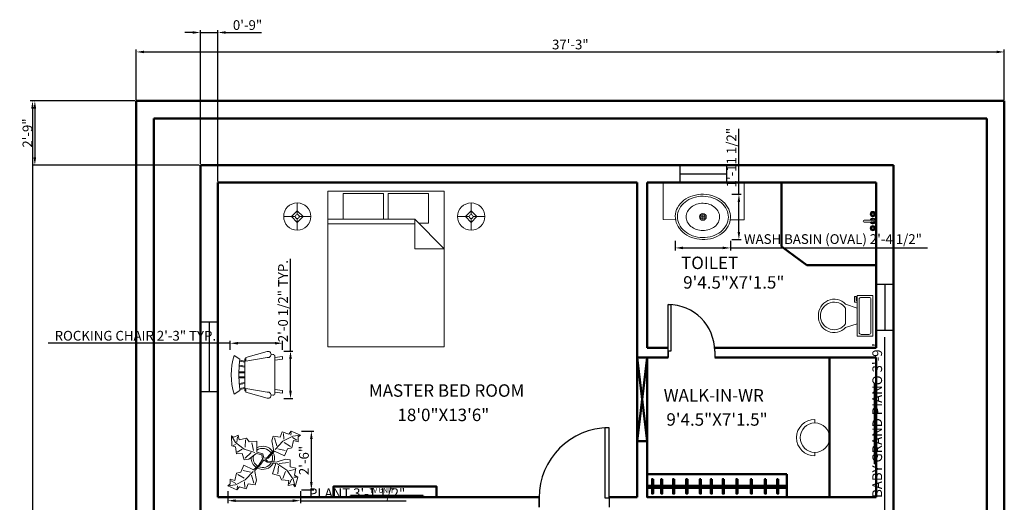
# Model space of a CAD drawing. Units: inches. Extents: x 116541 to 117938, y 135634 to 136328.
# Tile 9 of 9: x 117394 to 117902, y 136080 to 136328. Entities that reach past the tile are written whole.
import ezdxf

# ---------------------------------------------------------------- set-up
doc = ezdxf.new("R2010")
doc.units = ezdxf.units.IN
for name, color, linetype, lineweight in [('A-ANNO-DIMS', 2, 'Continuous', 18), ('A-ANNO-TEXT', 7, 'Continuous', 25), ('A-AREA-IDEN', 3, 'Continuous', 25), ('A-DOOR', 4, 'Continuous', 25), ('A-FLOR-FIXT', 9, 'Continuous', 18), ('A-FURN', 8, 'Continuous', 18), ('A-GLAZ', 1, 'Continuous', 25), ('A-WALL', 7, 'Continuous', 50)]:
    doc.layers.add(name, color=color, linetype=linetype, lineweight=lineweight)
doc.styles.get("Standard").update_dxf_attribs({"font": 'arial.ttf'})
doc.dimstyles.new('ISO-25', dxfattribs={"dimtxt": 5, "dimasz": 4, "dimexe": 1.25, "dimexo": 0.625, "dimtad": 1, "dimdec": 3, "dimlunit": 3, "dimtxsty": 'Standard', "dimcen": 2.5, "dimadec": 0, "dimazin": 0, "dimtfac": 1, "dimtdec": 3, "dimtmove": 0, "dimatfit": 3, "dimfxl": 1, "dimarcsym": 0})

# ---------------------------------------------------------------- blocks, each defined once
blk = doc.blocks.new('Plant - Rubber or Philodendron')
for p, q in [((-16.2005, 11.4774), (-13.9899, 8.1064)), ((-16.2005, 11.4774), (-14.8639, 10.7964)), ((-16.0159, 6.3329), (-16.2005, 11.4774)), ((-14.8639, 10.7964), (-12.6195, 11.8975)), ((-13.3174, 8.325), (-13.0735, 11.0065)), ((-12.6195, 11.8975), (-12.1909, 9.4345)), ((-12.1909, 9.4345), (-8.3829, 10.3)), ((-8.3829, 10.3), (-7.0549, 8.501)), ((4.6914, 8.8812), (5.3859, 11.2828)), ((5.3859, 11.2828), (8.8871, 10.7908)), ((5.9878, 10.4842), (7.1971, 6.3869)), ((8.8871, 10.7908), (9.9809, 13.4933)), ((9.9809, 13.4933), (13.3837, 12.301)), ((15.3859, 11.3055), (10.3916, 8.7942)), ((10.5828, 12.6946), (10.8893, 9.7953)), ((13.3837, 12.301), (14.68, 13.9039)), ((14.5816, 13.2037), (14.3848, 11.8033)), ((14.68, 13.9039), (19.3848, 11.8146)), ((15.2875, 10.6053), (17.5907, 9.2105)), ((19.3848, 11.8146), (15.3859, 11.3055)), ((19.3848, 11.8146), (18.1868, 10.9119)), ((18.1868, 10.9119), (18.1925, 8.4119)), ((-14.0069, 5.8704), (-16.0159, 6.3329)), ((-15.3434, 6.5514), (-13.9984, 6.9884)), ((-13.5868, 2.2894), (-14.0069, 5.8704)), ((-13.9899, 8.1064), (-9.5434, 4.7185)), ((-8.8369, 9.409), (-9.0894, 5.6095)), ((-7.0549, 8.501), (-3.0284, 8.6941)), ((-4.8529, 4.012), (-5.7184, 7.82)), ((-3.0284, 8.6941), (-3.0709, 3.1041)), ((4.6914, 8.8812), (5.5014, 4.4831)), ((10.3916, 8.7942), (6.2847, 4.4028)), ((14.2977, 6.1031), (10.9934, 7.9956)), ((14.8995, 5.3044), (12.7005, 4.8994)), ((15.7909, 9.1065), (14.8995, 5.3044)), ((18.1925, 8.4119), (15.7909, 9.1065)), ((-10.6784, 2.491), (-13.5868, 2.2894)), ((-13.1329, 3.1804), (-10.6614, 4.727)), ((-9.5858, -0.8715), (-10.6784, 2.491)), ((-9.5434, 4.7185), (-4.1917, 2.9888)), ((-9.1318, 0.0195), (-5.9793, 2.9025)), ((-7.1228, -0.443), (-3.5248, 2.2131)), ((-3.5248, 2.2131), (-3.3011, 2.4355)), ((-3.3011, 2.4355), (-0.5306, 1.7947)), ((-3.0709, 3.1041), (0.0797, 2.3163)), ((-0.5306, 1.7947), (-0.2255, -0.5527)), ((-0.5306, 1.7947), (-0.5306, 1.7947)), ((0.0797, 2.3163), (0.4866, -0.031)), ((0.4866, -0.031), (2.1141, 0.2298)), ((2.1141, 0.2298), (5.4346, 3.9146)), ((6.1032, 3.6844), (2.8262, -0.031)), ((5.4346, 3.9146), (5.5014, 4.4831)), ((11.1089, 1.1958), (6.1032, 3.6844)), ((7.7005, 4.8881), (11.5025, 3.9967)), ((12.7005, 4.8994), (11.1089, 1.1958)), ((-11.3237, -7.2629), (-9.7321, -3.5593)), ((-9.7321, -3.5593), (-4.7264, -6.0479)), ((-7.1228, -0.443), (-9.5858, -0.8715)), ((-2.019, -3.6148), (-4.7264, -6.0479)), ((-4.0579, -6.2781), (-0.9375, -3.1608)), ((-2.019, -3.6148), (-0.2255, -0.5527)), ((-0.9375, -3.1608), (0.5883, -0.8135)), ((0.5883, -0.8135), (2.2447, -2.0916)), ((2.8262, -0.031), (1.3003, -0.5527)), ((1.3003, -0.5527), (2.4193, -1.4655)), ((2.2447, -2.0916), (6.7108, -2.6626)), ((2.4193, -1.4655), (6.895, -2.1175)), ((4.943, -7.9659), (6.7108, -2.6626)), ((11.6605, -0.5413), (6.895, -2.1175)), ((12.3677, -6.1981), (7.219, -2.6772)), ((8.125, -4.0768), (7.7715, -7.9659)), ((8.3544, -2.7453), (13.1973, -2.1704)), ((11.6605, -0.5413), (14.1354, -0.8948)), ((14.1354, -0.8948), (14.1354, -4.4304)), ((14.1354, -4.4304), (16.9638, -5.1375)), ((-14.4141, -11.4699), (-13.5228, -7.6679)), ((-13.5228, -7.6679), (-11.3237, -7.2629)), ((-12.921, -8.4665), (-9.6166, -10.359)), ((-6.3237, -7.2516), (-10.1257, -6.3602)), ((-9.0148, -11.1577), (-4.9047, -6.8122)), ((-4.611, -12.8477), (-5.8203, -8.7504)), ((-4.1246, -6.8466), (-4.0579, -6.2781)), ((-3.3146, -11.2447), (-4.1246, -6.8466)), ((8.8321, -9.0266), (4.943, -7.9659)), ((9.5392, -11.1479), (8.8321, -9.0266)), ((10.2463, -10.4408), (11.6605, -6.9053)), ((15.5496, -10.7943), (12.3677, -6.1981)), ((16.2567, -5.8446), (13.4283, -6.5517)), ((17.3174, -9.7337), (15.9032, -9.7337)), ((16.9638, -5.1375), (16.2567, -8.673)), ((16.2567, -8.673), (18.0245, -9.7337)), ((18.0245, -9.7337), (16.6103, -14.6834)), ((-18.008, -14.1781), (-16.8101, -13.2754)), ((-18.008, -14.1781), (-14.0091, -13.669)), ((-13.3032, -16.2674), (-18.008, -14.1781)), ((-16.8157, -10.7754), (-14.4141, -11.4699)), ((-16.8101, -13.2754), (-16.8157, -10.7754)), ((-13.9107, -12.9688), (-16.2139, -11.574)), ((-14.0091, -13.669), (-9.0148, -11.1577)), ((-12.0069, -14.6645), (-13.3032, -16.2674)), ((-13.2048, -15.5672), (-13.008, -14.1668)), ((-8.6042, -15.8568), (-12.0069, -14.6645)), ((-9.206, -15.0581), (-9.5126, -12.1588)), ((-7.5103, -13.1543), (-8.6042, -15.8568)), ((-4.0092, -13.6463), (-7.5103, -13.1543)), ((-3.3146, -11.2447), (-4.0092, -13.6463)), ((13.4283, -11.5015), (9.5392, -11.1479)), ((13.0748, -13.9763), (13.4283, -11.5015)), ((15.5496, -13.6228), (13.0748, -13.9763)), ((14.8425, -10.7943), (13.7819, -13.2692)), ((16.6103, -14.6834), (15.5496, -10.7943)), ((16.6103, -14.6834), (15.5496, -13.6228))]:
    blk.add_line(p, q)
for centre, radius, start, end in [((0, 0), 6.1275, 34.37569, 120.1028), ((0.0308, 0.1664), 6, 178.6147, 235.1169), ((0.0308, 0.1664), 5, 168.1647, 238.6725), ((-0.0601, -0.2075), 5.2461, 33.82192, 124.9414), ((-0.2664, 0.1682), 5.2775, 338.4094, 20.03007), ((-0.098, 0.1364), 6.1288, 341.2017, 26.09184), ((-0.0234, 0.3825), 6.1492, 242.5812, 331.2714), ((-0.1102, 0.4886), 5.2883, 247.3711, 327.472)]:
    blk.add_arc(centre, radius, start, end)
blk = doc.blocks.new('Bed - Queen')
for p, q in [((0, -80.00003), (0, 0)), ((0, 0), (59.99999, 0)), ((59.99999, 0), (59.99999, -80.00003)), ((7.99999, -1.2), (28.79998, -1.2)), ((7.99999, -14.4), (7.99999, -1.2)), ((28.79998, -1.2), (28.79998, -14.4)), ((31.19999, -1.2), (51.99999, -1.2)), ((31.19999, -14.4), (31.19999, -1.2)), ((51.99999, -1.2), (51.99999, -16.4)), ((0, -14.4), (44.8, -14.4)), ((59.99999, -29.6), (44.8, -14.4)), ((44.8, -14.4), (44.8, -29.6)), ((44.8, -16.8), (0, -16.8)), ((51.99999, -16.4), (46.79936, -16.4)), ((44.8, -29.6), (59.99999, -29.6)), ((59.99999, -80.00003), (0, -80.00003))]:
    blk.add_line(p, q)
blk = doc.blocks.new('*U45')
for p, q in [((9.5, -6), (9.5, -2)), ((-10, -8.5), (-8, -8.5)), ((-10, -9.5), (-10, -8.5)), ((-7, -9.5), (-10, -9.5)), ((-8, -8.5), (-8, -8)), ((-7, -8), (-7, -9.5)), ((-4, -8), (-6, -14)), ((4, -8), (6, -14)), ((4, -14), (-4, -14))]:
    blk.add_line(p, q)
blk.add_lwpolyline([(10.5, -8), (10.5, 0), (-10.5, 0), (-10.5, -8)], close=True)
for points in [[(-9.5, -2), (-9.5, -6)], [(8.5, -1), (-8.5, -1)], [(-8.5, -7), (8.5, -7)]]:
    blk.add_lwpolyline(points)
for centre, radius, start, end in [((-8.625, -1.875), 0.8839, 81.8699, 188.1301), ((8.625, -1.875), 0.8839, 351.8699, 98.1301), ((-8.625, -6.125), 0.8839, 171.869898, 278.1301), ((8.625, -6.125), 0.8839, 261.8699, 8.1301), ((-0.4772, -19.9188), 8.0953, 133.01722, 273.38), ((0.0374, -19.8731), 7.127, 124.50543, 269.7), ((-0.0373, -19.8731), 7.127, 270.3, 55.4946), ((0.4773, -19.9188), 8.0953, 266.62, 46.9828)]:
    blk.add_arc(centre, radius, start, end)
blk = doc.blocks.new('Faucet - Bathroom top')
for p, q in [((-4.107, 0.125), (-4.375, 0.125)), ((-3.75, 0.4788), (-3.75, 0.75)), ((-3.5, 0.482), (-3.5, 0.75)), ((-3.1461, 0.125), (-2.875, 0.125)), ((3.143, 0.125), (2.875, 0.125)), ((3.5, 0.4788), (3.5, 0.75)), ((3.75, 0.482), (3.75, 0.75)), ((4.1039, 0.125), (4.375, 0.125)), ((-4.1039, -0.125), (-4.375, -0.125)), ((-3.75, -0.4821), (-3.75, -0.75)), ((-3.5, -0.4789), (-3.5, -0.75)), ((-3.143, -0.125), (-2.875, -0.125)), ((-0.5, -0.8639), (-0.5, -4.5)), ((0.5, -4.5), (0.5, -0.8631)), ((3.1461, -0.125), (2.875, -0.125)), ((3.5, -0.4821), (3.5, -0.75)), ((3.75, -0.4789), (3.75, -0.75)), ((4.107, -0.125), (4.375, -0.125))]:
    blk.add_line(p, q)
for centre, radius in [((-3.625, 0), 1.375), ((-4.625, 0), 0.2795), ((-3.625, 0), 0.5), ((-3.625, 1), 0.2795), ((-2.625, 0), 0.2795), ((0, 0), 0.5), ((3.625, 0), 1.375), ((2.625, 0), 0.2795), ((3.625, 0), 0.5), ((3.625, 1), 0.2795), ((4.625, 0), 0.2795), ((-3.625, -1), 0.2795), ((3.625, -1), 0.2795)]:
    blk.add_circle(centre, radius)
for centre, radius, start, end in [((-3.625, 0), 1, 105.2407, 164.2093), ((-3.625, 0), 1, 16.44125, 74.07887), ((0, 0), 1.5, 289.6514, 250.3603), ((0, 0), 1, 300.3431, 239.7554), ((3.625, 0), 1, 106.12, 164.0884), ((3.625, 0), 1, 16.23422, 73.90469), ((-3.625, 0), 1, 196.2342, 253.9047), ((-3.625, 0), 1, 286.12, 344.0884), ((0, -4.5), 0.5, 180, 0), ((3.625, 0), 1, 196.4413, 254.0789), ((3.625, 0), 1, 285.2407, 344.2093)]:
    blk.add_arc(centre, radius, start, end)
blk = doc.blocks.new('Sink - Oval top')
for p, q in [((-1, 0), (1, 0)), ((0, 1), (0, -1))]:
    blk.add_line(p, q)
for points in [[(-12.23, 0.39, 0.117634), (-11.46, -3.36, 0.104469), (-8.88, -6.8, 0.090016), (-5.08, -9.07, 0.08192), (-0.32, -10.02, 0.08192), (4.49, -9.38, 0.090016), (8.42, -7.36, 0.104469), (11.22, -4.09, 0.117634), (12.23, -0.39, 0.117634), (11.46, 3.36, 0.104469), (8.88, 6.8, 0.090016), (5.08, 9.07, 0.08192), (0.32, 10.02, 0.08192), (-4.49, 9.38, 0.090016), (-8.42, 7.36, 0.104469), (-11.22, 4.09, 0.117634)], [(-11.29, 0.16, 0.118622), (-10.52, -3.25, 0.104678), (-8.07, -6.36, 0.089562), (-4.54, -8.37, 0.081185), (-0.13, -9.15, 0.081185), (4.3, -8.49, 0.089562), (7.89, -6.58, 0.104678), (10.42, -3.55, 0.118622), (11.29, -0.16, 0.118622), (10.52, 3.25, 0.104678), (8.07, 6.36, 0.089562), (4.54, 8.37, 0.081185), (0.13, 9.15, 0.081185), (-4.3, 8.49, 0.089562), (-7.89, 6.58, 0.104678), (-10.42, 3.55, 0.118622)], [(-7.42, 0.08, 0.118283), (-6.91, -2.17, 0.104607), (-5.29, -4.21, 0.089718), (-2.97, -5.53, 0.081436), (-0.07, -6.04, 0.081436), (2.84, -5.59, 0.089718), (5.2, -4.33, 0.104607), (6.86, -2.32, 0.118283), (7.42, -0.08, 0.118283), (6.91, 2.17, 0.104607), (5.29, 4.21, 0.089718), (2.97, 5.53, 0.081436), (0.07, 6.04, 0.081436), (-2.84, 5.59, 0.089718), (-5.2, 4.33, 0.104607), (-6.86, 2.32, 0.118283)]]:
    blk.add_lwpolyline(points, format="xyb", close=True)
for radius in [1.5, 1]:
    blk.add_circle((0, 0), radius)
blk = doc.blocks.new('Lamp - Table')
for p, q in [((0, 7), (0, 1)), ((-1, 0), (-7, 0)), ((0, 3), (-3, 0)), ((-3, 0), (0, -3)), ((3, 0), (0, 3)), ((0, -3), (3, 0)), ((1, 0), (7, 0)), ((0, -1), (0, -7))]:
    blk.add_line(p, q)
for radius in [7, 1]:
    blk.add_circle((0, 0), radius)
blk = doc.blocks.new('*U48')
for p, q in [((-750, 0), (-750, -100)), ((0, 0), (0, -100))]:
    blk.add_line(p, q)
blk.add_lwpolyline([(0, 0), (0, 750), (-43.75, 750), (-43.75, 0)], close=True)
blk.add_arc((0, 0), 750, 90, 180)
blk = doc.blocks.new('*U47')
for p, q in [((0, 0), (0, -100)), ((750, 0), (750, -100))]:
    blk.add_line(p, q)
blk.add_lwpolyline([(0, 0), (0, 750), (43.75, 750), (43.75, 0)], close=True)
blk.add_arc((0, 0), 750, 0, 90)
blk = doc.blocks.new('Chair - Rocking')
for p, q in [((-8, -4.5), (-10, -1.5)), ((-7.5, -4.5), (-7, -7)), ((-6.5, -7), (-7.02225, -4.43)), ((-4.5, -7), (-4.96674, -4.19951)), ((-4, -7), (-4.40532, -4.16272)), ((-1.5, -4.05012), (-1.5, -7)), ((-1, -7), (-1, -4.05012)), ((1, -7), (1, -4.04655)), ((1.5, -4.05012), (1.5, -7)), ((4, -7), (4.40187, -4.18694)), ((4.5, -7), (4.96761, -4.19437)), ((6.5, -7), (7, -4.4057)), ((7.5, -4.5), (7, -7)), ((8, -4.5), (10, -1.5)), ((-9, -7.5), (-12, -18.49999)), ((-7, -7.5), (-9, -7.5)), ((-9, -18.49999), (-7, -7.5)), ((-8.23428, -6.99939), (-8.3093, -7.47958)), ((-8.23041, -7), (8.23915, -7)), ((7, -7.5), (9, -7.5)), ((9, -18.49999), (7, -7.5)), ((8.31071, -7.48854), (8.23449, -7.00073)), ((9, -7.5), (12, -18.49999)), ((-10.36644, -20.64523), (-10.5, -21.49999)), ((-9, -22.49999), (-9.5, -26.49999)), ((0, -22.49999), (-9.5, -22.49999)), ((-8, -26.49999), (-7.5, -22.49999)), ((0, -22.49999), (9.5, -22.49999)), ((8, -26.49999), (7.5, -22.49999)), ((9, -22.49999), (9.5, -26.49999)), ((10.5, -21.49999), (10.3575, -20.58798)), ((-9.5, -26.49999), (-8, -26.49999)), ((9.5, -26.49999), (8, -26.49999))]:
    blk.add_line(p, q)
for centre, radius, start, end in [((0, -34.08333), 34.08333, 72.93847, 107.0615), ((0, -68.25004), 64.25, 93.92211, 97.15267), ((0, -68.25004), 64.25, 82.84733, 93.92211), ((-10.5, -18.99999), 1.58114, 161.5651, 18.43495), ((10.5, -18.99999), 1.58114, 161.5651, 18.43495), ((-9.5, -21.49999), 1, 180, 270), ((9.5, -21.49999), 1, 270, 0)]:
    blk.add_arc(centre, radius, start, end)
blk = doc.blocks.new('*D54')
at = {"layer": 'A-ANNO-DIMS', "color": 0, "lineweight": -2, "transparency": 16777216}
for p, q in [((117453.9, 136286.5), (117399.8, 136286.5)), ((117401.05, 136282.5), (117401.05, 135738.5)), ((117453.9, 135734.5), (117399.8, 135734.5))]:
    blk.add_line(p, q, dxfattribs=at)
at = {"layer": 'A-ANNO-DIMS', "color": 0, "transparency": 16777216}
for points in [[(117400.38, 136282.5), (117401.71, 136282.5), (117401.05, 136286.5)], [(117400.38, 135738.5), (117401.71, 135738.5), (117401.05, 135734.5)]]:
    blk.add_solid(points, dxfattribs=at)
at = {"layer": 'Defpoints', "color": 0, "transparency": 16777216}
for p in [(117454.52, 136286.5), (117401.05, 135734.5), (117454.52, 135734.5)]:
    blk.add_point(p, dxfattribs=at)
at = {"layer": 'A-ANNO-DIMS', "color": 0, "transparency": 16777216, "insert": (117397.87, 136010.5), "char_height": 5, "attachment_point": 5, "rotation": 90}
blk.add_mtext("46'", dxfattribs=at)
blk = doc.blocks.new('*D55')
at = {"layer": 'A-ANNO-DIMS', "color": 0, "lineweight": -2, "transparency": 16777216}
for p, q in [((117454.52, 136287.13), (117454.52, 136312.99)), ((117458.52, 136311.74), (117897.52, 136311.74)), ((117901.52, 136287.13), (117901.52, 136312.99))]:
    blk.add_line(p, q, dxfattribs=at)
at = {"layer": 'A-ANNO-DIMS', "color": 0, "transparency": 16777216}
for points in [[(117458.52, 136312.41), (117458.52, 136311.08), (117454.52, 136311.74)], [(117897.52, 136312.41), (117897.52, 136311.08), (117901.52, 136311.74)]]:
    blk.add_solid(points, dxfattribs=at)
at = {"layer": 'Defpoints', "color": 0, "transparency": 16777216}
for p in [(117901.52, 136311.74), (117454.52, 136286.5), (117901.52, 136286.5)]:
    blk.add_point(p, dxfattribs=at)
at = {"layer": 'A-ANNO-DIMS', "color": 0, "transparency": 16777216, "insert": (117678.02, 136314.92), "char_height": 5, "attachment_point": 5}
blk.add_mtext('37\'-3"', dxfattribs=at)
blk = doc.blocks.new('WASH-BASIN')
for p, q in [((7.56, 17), (7.56, 18.87)), ((7.56, 0), (7.56, 1.87))]:
    blk.add_line(p, q)
blk.add_circle((7.56, 9.43), 7.56)
blk.add_arc((7.56, 9.43), 9.43, 270, 90)
blk = doc.blocks.new('*D58')
at = {"layer": 'A-ANNO-DIMS', "color": 0, "lineweight": -2, "transparency": 16777216}
for p, q in [((117501.66, 136085.74), (117501.66, 136079.51)), ((117539.05, 136085.74), (117539.05, 136079.51)), ((117505.66, 136080.76), (117535.05, 136080.76)), ((117539.05, 136080.76), (117593.45, 136080.76))]:
    blk.add_line(p, q, dxfattribs=at)
at = {"layer": 'A-ANNO-DIMS', "color": 0, "transparency": 16777216}
for points in [[(117505.66, 136081.43), (117505.66, 136080.09), (117501.66, 136080.76)], [(117535.05, 136081.43), (117535.05, 136080.09), (117539.05, 136080.76)]]:
    blk.add_solid(points, dxfattribs=at)
at = {"layer": 'Defpoints', "color": 0, "transparency": 16777216}
for p in [(117501.66, 136086.37), (117539.05, 136086.37), (117539.05, 136080.76)]:
    blk.add_point(p, dxfattribs=at)
at = {"layer": 'A-ANNO-DIMS', "color": 0, "transparency": 16777216, "insert": (117568.25, 136083.97), "char_height": 5, "attachment_point": 5}
blk.add_mtext('PLANT 3\'-1 1/2"', dxfattribs=at)
blk = doc.blocks.new('*D59')
at = {"layer": 'A-ANNO-DIMS', "color": 0, "lineweight": -2, "transparency": 16777216}
for p, q in [((117539.67, 136116.54), (117545.91, 136116.54)), ((117544.66, 136090.37), (117544.66, 136112.54)), ((117539.67, 136086.37), (117545.91, 136086.37))]:
    blk.add_line(p, q, dxfattribs=at)
at = {"layer": 'A-ANNO-DIMS', "color": 0, "transparency": 16777216}
for points in [[(117543.99, 136112.54), (117545.32, 136112.54), (117544.66, 136116.54)], [(117543.99, 136090.37), (117545.32, 136090.37), (117544.66, 136086.37)]]:
    blk.add_solid(points, dxfattribs=at)
at = {"layer": 'Defpoints', "color": 0, "transparency": 16777216}
for p in [(117539.05, 136116.54), (117544.66, 136116.54), (117539.05, 136086.37)]:
    blk.add_point(p, dxfattribs=at)
at = {"layer": 'A-ANNO-DIMS', "color": 0, "transparency": 16777216, "insert": (117541.48, 136101.45), "char_height": 5, "attachment_point": 5, "rotation": 90}
blk.add_mtext('2\'-6"', dxfattribs=at)
blk = doc.blocks.new('*D66')
at = {"layer": 'A-ANNO-DIMS', "color": 0, "lineweight": -2, "transparency": 16777216}
for p, q in [((117732.04, 136214.52), (117732.04, 136209.61)), ((117760.56, 136214.52), (117760.56, 136209.61)), ((117736.04, 136210.86), (117756.56, 136210.86)), ((117760.56, 136210.86), (117861.98, 136210.86))]:
    blk.add_line(p, q, dxfattribs=at)
at = {"layer": 'A-ANNO-DIMS', "color": 0, "transparency": 16777216}
for points in [[(117736.04, 136211.53), (117736.04, 136210.2), (117732.04, 136210.86)], [(117756.56, 136211.53), (117756.56, 136210.2), (117760.56, 136210.86)]]:
    blk.add_solid(points, dxfattribs=at)
at = {"layer": 'Defpoints', "color": 0, "transparency": 16777216}
for p in [(117732.04, 136215.14), (117760.56, 136215.14), (117760.56, 136210.86)]:
    blk.add_point(p, dxfattribs=at)
at = {"layer": 'A-ANNO-DIMS', "color": 0, "transparency": 16777216, "insert": (117813.27, 136214.77), "char_height": 5, "attachment_point": 5}
blk.add_mtext('WASH BASIN (OVAL) 2\'-4 1/2"', dxfattribs=at)
blk = doc.blocks.new('*D67')
at = {"layer": 'A-ANNO-DIMS', "color": 0, "lineweight": -2, "transparency": 16777216}
for p, q in [((117764.84, 136238.53), (117764.84, 136272.14)), ((117761.19, 136238.53), (117766.09, 136238.53)), ((117764.84, 136219.14), (117764.84, 136234.53)), ((117761.19, 136215.14), (117766.09, 136215.14))]:
    blk.add_line(p, q, dxfattribs=at)
at = {"layer": 'A-ANNO-DIMS', "color": 0, "transparency": 16777216}
for points in [[(117764.17, 136234.53), (117765.5, 136234.53), (117764.84, 136238.53)], [(117764.17, 136219.14), (117765.5, 136219.14), (117764.84, 136215.14)]]:
    blk.add_solid(points, dxfattribs=at)
at = {"layer": 'Defpoints', "color": 0, "transparency": 16777216}
for p in [(117760.56, 136238.53), (117764.84, 136238.53), (117760.56, 136215.14)]:
    blk.add_point(p, dxfattribs=at)
at = {"layer": 'A-ANNO-DIMS', "color": 0, "transparency": 16777216, "insert": (117761.63, 136257.33), "char_height": 5, "attachment_point": 5, "rotation": 90}
blk.add_mtext('1\'-11 1/2"', dxfattribs=at)
blk = doc.blocks.new('*D72')
at = {"layer": 'A-ANNO-DIMS', "color": 0, "lineweight": -2, "transparency": 16777216}
for p, q in [((117502.87, 136161.81), (117409.19, 136161.81)), ((117502.87, 136158.38), (117502.87, 136163.06)), ((117525.87, 136161.81), (117506.87, 136161.81)), ((117529.87, 136158.38), (117529.87, 136163.06))]:
    blk.add_line(p, q, dxfattribs=at)
at = {"layer": 'A-ANNO-DIMS', "color": 0, "transparency": 16777216}
for points in [[(117506.87, 136162.48), (117506.87, 136161.14), (117502.87, 136161.81)], [(117525.87, 136162.48), (117525.87, 136161.14), (117529.87, 136161.81)]]:
    blk.add_solid(points, dxfattribs=at)
at = {"layer": 'Defpoints', "color": 0, "transparency": 16777216}
for p in [(117502.87, 136161.81), (117502.87, 136157.76), (117529.87, 136157.76)]:
    blk.add_point(p, dxfattribs=at)
at = {"layer": 'A-ANNO-DIMS', "color": 0, "transparency": 16777216, "insert": (117454.03, 136165.02), "char_height": 5, "attachment_point": 5}
blk.add_mtext('ROCKING CHAIR 2\'-3" TYP.', dxfattribs=at)
blk = doc.blocks.new('*D73')
at = {"layer": 'A-ANNO-DIMS', "color": 0, "lineweight": -2, "transparency": 16777216}
for p, q in [((117533.92, 136157.76), (117533.92, 136205.22)), ((117530.49, 136157.76), (117535.17, 136157.76)), ((117533.92, 136137.32), (117533.92, 136153.76)), ((117530.49, 136133.32), (117535.17, 136133.32))]:
    blk.add_line(p, q, dxfattribs=at)
at = {"layer": 'A-ANNO-DIMS', "color": 0, "transparency": 16777216}
for points in [[(117533.25, 136153.76), (117534.59, 136153.76), (117533.92, 136157.76)], [(117533.25, 136137.32), (117534.59, 136137.32), (117533.92, 136133.32)]]:
    blk.add_solid(points, dxfattribs=at)
at = {"layer": 'Defpoints', "color": 0, "transparency": 16777216}
for p in [(117529.87, 136157.76), (117533.92, 136157.76), (117529.87, 136133.32)]:
    blk.add_point(p, dxfattribs=at)
at = {"layer": 'A-ANNO-DIMS', "color": 0, "transparency": 16777216, "insert": (117530.71, 136183.49), "char_height": 5, "attachment_point": 5, "rotation": 90}
blk.add_mtext('2\'-0 1/2" TYP.', dxfattribs=at)
blk = doc.blocks.new('*D96')
at = {"layer": 'A-ANNO-DIMS', "color": 0, "lineweight": -2, "transparency": 16777216}
for p, q in [((117839.93, 136075.15), (117839.93, 136164.88)), ((117833.8, 136075.15), (117841.18, 136075.15)), ((117839.93, 136034.11), (117839.93, 136071.15)), ((117833.8, 136030.11), (117841.18, 136030.11))]:
    blk.add_line(p, q, dxfattribs=at)
at = {"layer": 'A-ANNO-DIMS', "color": 0, "transparency": 16777216}
for points in [[(117839.26, 136071.15), (117840.6, 136071.15), (117839.93, 136075.15)], [(117839.26, 136034.11), (117840.6, 136034.11), (117839.93, 136030.11)]]:
    blk.add_solid(points, dxfattribs=at)
at = {"layer": 'Defpoints', "color": 0, "transparency": 16777216}
for p in [(117833.18, 136075.15), (117839.93, 136075.15), (117833.18, 136030.11)]:
    blk.add_point(p, dxfattribs=at)
at = {"layer": 'A-ANNO-DIMS', "color": 0, "transparency": 16777216, "insert": (117836.72, 136122.01), "char_height": 5, "attachment_point": 5, "rotation": 90}
blk.add_mtext('BABY GRAND PIANO 3\'-9"', dxfattribs=at)
blk = doc.blocks.new('*D101')
at = {"layer": 'A-ANNO-DIMS', "color": 0, "lineweight": -2, "transparency": 16777216}
for p, q in [((117453.9, 136286.5), (117401.02, 136286.5)), ((117402.27, 136282.5), (117402.27, 136257.5)), ((117486.9, 136253.5), (117401.02, 136253.5))]:
    blk.add_line(p, q, dxfattribs=at)
at = {"layer": 'A-ANNO-DIMS', "color": 0, "transparency": 16777216}
for points in [[(117401.6, 136282.5), (117402.94, 136282.5), (117402.27, 136286.5)], [(117401.6, 136257.5), (117402.94, 136257.5), (117402.27, 136253.5)]]:
    blk.add_solid(points, dxfattribs=at)
at = {"layer": 'Defpoints', "color": 0, "transparency": 16777216}
for p in [(117454.52, 136286.5), (117402.27, 136253.5), (117487.52, 136253.5)]:
    blk.add_point(p, dxfattribs=at)
at = {"layer": 'A-ANNO-DIMS', "color": 0, "transparency": 16777216, "insert": (117399.09, 136270), "char_height": 5, "attachment_point": 5, "rotation": 90}
blk.add_mtext('2\'-9"', dxfattribs=at)
blk = doc.blocks.new('*D103')
at = {"layer": 'A-ANNO-DIMS', "color": 0, "lineweight": -2, "transparency": 16777216}
for p, q in [((117483.52, 136321.75), (117479.52, 136321.75)), ((117487.52, 136254.13), (117487.52, 136323)), ((117487.52, 136321.75), (117496.52, 136321.75)), ((117496.52, 136245.13), (117496.52, 136323)), ((117500.52, 136321.75), (117519.06, 136321.75))]:
    blk.add_line(p, q, dxfattribs=at)
at = {"layer": 'A-ANNO-DIMS', "color": 0, "transparency": 16777216}
for points in [[(117483.52, 136322.42), (117483.52, 136321.09), (117487.52, 136321.75)], [(117500.52, 136322.42), (117500.52, 136321.09), (117496.52, 136321.75)]]:
    blk.add_solid(points, dxfattribs=at)
at = {"layer": 'Defpoints', "color": 0, "transparency": 16777216}
for p in [(117496.52, 136321.75), (117487.52, 136253.5), (117496.52, 136244.5)]:
    blk.add_point(p, dxfattribs=at)
at = {"layer": 'A-ANNO-DIMS', "color": 0, "transparency": 16777216, "insert": (117511.79, 136324.93), "char_height": 5, "attachment_point": 5}
blk.add_mtext('0\'-9"', dxfattribs=at)

msp = doc.modelspace()

# ---------------------------------------------------------------- linework, layer by layer
at = {"layer": 'A-DOOR'}
for points in [[(117728.4087, 136154.5034), (117728.4087, 136159.5034)], [(117661.9632, 136077.5034), (117661.9632, 136082.5034)], [(117697.9632, 136082.5034), (117697.9632, 136077.5034)]]:
    msp.add_lwpolyline(points, dxfattribs=at)
at = {"layer": 'A-FLOR-FIXT'}
for p, q in [((117725.903, 136244.5034), (117725.903, 136225.4134)), ((117767.5729, 136225.4031), (117767.5729, 136244.5034)), ((117725.903, 136225.4134), (117732.2209, 136225.3929)), ((117760.4303, 136225.4031), (117767.5729, 136225.4031))]:
    msp.add_line(p, q, dxfattribs=at)
at = {"layer": 'A-GLAZ'}
for p, q in [((117734.515, 136249.0034), (117758.515, 136249.0034)), ((117840.0209, 136192.2849), (117840.0209, 136168.2849)), ((117492.0209, 136172.7898), (117492.0209, 136136.7898)), ((117834.5209, 136141.1488), (117834.5209, 136099.7563)), ((117835.5209, 136141.1488), (117834.5209, 136141.1488)), ((117835.5209, 136141.1488), (117835.5209, 136099.7563)), ((117835.5209, 136099.7563), (117834.5209, 136099.7563))]:
    msp.add_line(p, q, dxfattribs=at)
for points in [[(117734.515, 136244.5034), (117734.515, 136253.5034), (117758.515, 136253.5034), (117758.515, 136244.5034)], [(117835.5209, 136192.2849), (117844.5209, 136192.2849), (117844.5209, 136168.2849), (117835.5209, 136168.2849)], [(117487.5209, 136172.7898), (117496.5209, 136172.7898), (117496.5209, 136136.7898), (117487.5209, 136136.7898)]]:
    msp.add_lwpolyline(points, close=True, dxfattribs=at)
at = {"layer": 'A-WALL'}
for p, q in [((117454.5209, 136286.5034), (117454.5209, 135734.5034)), ((117454.5209, 136286.5034), (117871.5209, 136286.5034)), ((117871.5209, 136286.5034), (117901.5209, 136286.5034)), ((117901.5209, 136286.5034), (117901.5209, 135734.5034)), ((117463.5209, 136277.5034), (117463.5209, 135743.5034)), ((117463.5209, 136277.5034), (117871.5209, 136277.5034)), ((117871.5209, 136277.5034), (117892.5209, 136277.5034)), ((117892.5209, 136277.5034), (117892.5209, 136244.5034)), ((117487.5209, 136253.5034), (117487.5209, 135797.5034)), ((117844.5209, 136253.5034), (117487.5209, 136253.5034)), ((117844.5209, 135951.0034), (117844.5209, 136253.5034)), ((117496.5209, 136244.5034), (117712.5209, 136244.5034)), ((117496.5209, 136244.5034), (117496.5209, 136082.5034)), ((117712.5209, 136244.5034), (117496.5209, 136244.5034)), ((117712.5209, 136244.5034), (117712.5209, 136082.5034)), ((117835.5209, 136244.5034), (117717.5209, 136244.5034)), ((117717.5209, 136244.5034), (117717.5209, 136159.5034)), ((117717.5209, 136244.5034), (117835.5209, 136244.5034)), ((117786.6957, 136211.5469), (117786.6957, 136244.5034)), ((117835.5209, 136159.5034), (117835.5209, 136244.5034)), ((117892.5209, 136244.5034), (117892.5209, 135750.0323)), ((117799.8617, 136202.0034), (117786.6957, 136211.5469)), ((117799.8617, 136202.0034), (117786.6957, 136211.5469)), ((117835.5209, 136202.0034), (117799.8617, 136202.0034)), ((117728.4087, 136159.5034), (117717.5209, 136159.5034)), ((117835.5209, 136159.5034), (117752.3411, 136159.5034)), ((117712.5209, 136154.5034), (117717.5209, 136111.3198)), ((117712.5209, 136111.3198), (117717.5209, 136154.5034)), ((117728.4087, 136154.5034), (117712.5209, 136154.5034)), ((117717.5209, 136154.5034), (117717.5209, 136082.5034)), ((117835.5209, 136154.5034), (117752.4087, 136154.5034)), ((117811.5209, 136082.5034), (117811.5209, 136154.5034)), ((117835.5209, 136082.5034), (117835.5209, 136154.5034)), ((117717.5209, 136111.3198), (117712.5209, 136111.3198)), ((117717.5209, 136082.3634), (117717.5209, 136094.3634)), ((117717.5209, 136094.3634), (117789.5209, 136094.3634)), ((117789.5209, 136094.3634), (117789.5209, 136082.5034)), ((117717.5209, 136088.3634), (117789.5209, 136088.3634)), ((117717.5209, 136087.3634), (117789.5209, 136087.3634)), ((117661.9632, 136082.5034), (117496.5209, 136082.5034)), ((117564.7866, 136082.5034), (117564.7866, 136083.3016)), ((117564.7866, 136083.3016), (117602.1708, 136083.3016)), ((117602.1708, 136083.3016), (117602.1708, 136082.5034)), ((117712.5209, 136082.5034), (117697.9632, 136082.5034)), ((117835.5209, 136082.5034), (117717.5209, 136082.5034))]:
    msp.add_line(p, q, dxfattribs=at)
for points in [[(117720.6516, 136091.9252), (117720.6516, 136084.3953), (117720.1013, 136084.3953), (117720.1013, 136091.9252)], [(117725.3819, 136091.9252), (117725.3819, 136084.3953), (117724.8316, 136084.3953), (117724.8316, 136091.9252)], [(117731.5094, 136091.9252), (117731.5094, 136084.3953), (117730.9591, 136084.3953), (117730.9591, 136091.9252)], [(117738.2931, 136091.9252), (117738.2931, 136084.3953), (117737.7429, 136084.3953), (117737.7429, 136091.9252)], [(117745.2957, 136091.9252), (117745.2957, 136084.3953), (117744.7454, 136084.3953), (117744.7454, 136091.9252)], [(117750.9854, 136091.9252), (117750.9854, 136084.3953), (117750.4351, 136084.3953), (117750.4351, 136091.9252)], [(117757.1127, 136091.9252), (117757.1127, 136084.3953), (117756.5624, 136084.3953), (117756.5624, 136091.9252)], [(117764.1152, 136091.9252), (117764.1152, 136084.3953), (117763.5649, 136084.3953), (117763.5649, 136091.9252)], [(117771.5555, 136091.9252), (117771.5555, 136084.3953), (117771.0052, 136084.3953), (117771.0052, 136091.9252)], [(117778.7771, 136091.9252), (117778.7771, 136084.3953), (117778.2268, 136084.3953), (117778.2268, 136091.9252)], [(117785.1233, 136091.9252), (117785.1233, 136084.3953), (117784.573, 136084.3953), (117784.573, 136091.9252)], [(117556.0781, 136082.5034), (117609.0588, 136082.5034), (117609.0588, 136088.1091), (117556.0781, 136088.1091)]]:
    msp.add_lwpolyline(points, close=True, dxfattribs=at)

# ---------------------------------------------------------------- block references
at = {"layer": 'A-DOOR'}
for name, p, xscale, yscale, zscale in [('*U47', (117728.4087, 136157.7034), 0.0320000000000009, 0.0320000000000009, 0.0320000000000009), ('*U48', (117697.9632, 136082.3034), 0.0480000000000013, 0.0480000000000013, 0.0480000000000013)]:
    msp.add_blockref(name, p, dxfattribs=dict(at, xscale=xscale, yscale=yscale, zscale=zscale))
at = {"layer": 'A-FLOR-FIXT', "xscale": 1.161498081609967, "yscale": 1.161498081609967, "zscale": 1.161498081609967}
msp.add_blockref('Sink - Oval top', (117746.3023, 136226.8366), dxfattribs=at)
at = {"layer": 'A-FLOR-FIXT'}
for name, p, rotation in [('Faucet - Bathroom top', (117833.8124, 136224.6624), 270), ('WASH-BASIN', (117811.5207, 136122.6359), 180)]:
    msp.add_blockref(name, p, dxfattribs=dict(at, rotation=rotation))
at = {"layer": 'A-FURN'}
for name, p in [('Bed - Queen', (117553.0719, 136240.0373)), ('Lamp - Table', (117537.4034, 136227.0004)), ('Lamp - Table', (117626.9638, 136227.0004)), ('Plant - Rubber or Philodendron', (117519.6632, 136102.6365))]:
    msp.add_blockref(name, p, dxfattribs=at)
for name, p, rotation in [('*U45', (117833.815, 136175.8712), 270), ('Chair - Rocking', (117503.3694, 136145.5424), 90)]:
    msp.add_blockref(name, p, dxfattribs=dict(at, rotation=rotation))

# ---------------------------------------------------------------- texts
at = {"layer": 'A-ANNO-TEXT'}
msp.add_text('TV UNIT', height=2.48251, dxfattribs=at).set_placement((117574.5072, 136084.7386))
at = {"layer": 'A-AREA-IDEN'}
for s, height, p in [('TOILET', 6.40837, (117735.0574, 136199.9742)), ('9\'4.5"X7\'1.5"', 6.408368, (117736.1445, 136189.9189)), ('MASTER BED ROOM', 6.408368, (117574.3064, 136134.2549)), ('WALK-IN-WR', 6.40837, (117726.1099, 136131.7679)), ('18\'0"X13\'6"', 6.408368, (117589.019, 136121.7223)), ('9\'4.5"X7\'1.5"', 6.408368, (117727.5149, 136119.3595))]:
    msp.add_text(s, height=height, dxfattribs=at).set_placement(p)

# ---------------------------------------------------------------- dimensions: what is measured, and where the dimension line sits
at = {"layer": 'A-ANNO-DIMS'}
for base, p1, p2, override, picture, middle in [((117496.5209, 136321.7534), (117487.5209, 136253.5034), (117496.5209, 136244.5034), {"dimdec": 1, "dimlfac": 1, "dimrnd": 0, "dimzin": 1, "dimdsep": 46, "dimlunit": 4, "dimfrac": 2}, '*D103', (117511.7915, 136324.9313)), ((117901.5209, 136311.7433), (117454.5209, 136286.5034), (117901.5209, 136286.5034), {"dimclrd": 0, "dimclre": 0, "dimclrt": 0}, '*D55', (117678.0209, 136314.9229))]:
    dim = msp.add_linear_dim(base=base, p1=p1, p2=p2, dimstyle='ISO-25', override=override, dxfattribs=at)
    dim.commit()
    dim.dimension.update_dxf_attribs({"geometry": picture, "text_midpoint": middle})
for base, p1, p2, override, picture, middle in [((117401.0451, 135734.5034), (117454.5209, 136286.5034), (117454.5209, 135734.5034), {"dimclrd": 0, "dimclre": 0, "dimclrt": 0}, '*D54', (117397.8672, 136010.5034)), ((117402.2709, 136253.5034), (117454.5209, 136286.5034), (117487.5209, 136253.5034), {"dimdec": 1, "dimlfac": 1, "dimrnd": 0, "dimzin": 1, "dimdsep": 46, "dimlunit": 4, "dimfrac": 2}, '*D101', (117399.093, 136270.0034)), ((117764.8375, 136238.5309), (117760.5602, 136215.1423), (117760.5602, 136238.5309), {"dimdec": 1, "dimrnd": 0, "dimzin": 1, "dimlunit": 4, "dimfrac": 2}, '*D67', (117761.6273, 136257.334)), ((117544.657, 136116.5404), (117539.048, 136086.3691), (117539.048, 136116.5404), {"dimdec": 1, "dimrnd": 0, "dimzin": 1, "dimlunit": 4, "dimfrac": 2}, '*D59', (117541.4791, 136101.4548))]:
    dim = msp.add_linear_dim(base=base, p1=p1, p2=p2, angle=90, dimstyle='ISO-25', override=override, dxfattribs=at)
    dim.commit()
    dim.dimension.update_dxf_attribs({"geometry": picture, "text_midpoint": middle})
for base, p1, p2, text, picture, middle in [((117760.5602, 136210.8649), (117732.0443, 136215.1423), (117760.5602, 136215.1423), 'WASH BASIN (OVAL) <>', '*D66', (117813.2718, 136214.7693)), ((117539.048, 136080.7602), (117501.6552, 136086.3691), (117539.048, 136086.3691), 'PLANT <>', '*D58', (117568.2467, 136083.9722))]:
    dim = msp.add_linear_dim(base=base, p1=p1, p2=p2, text=text, dimstyle='ISO-25', override={"dimdec": 1, "dimrnd": 0, "dimzin": 1, "dimlunit": 4, "dimfrac": 2}, dxfattribs=at)
    dim.commit()
    dim.dimension.update_dxf_attribs({"geometry": picture, "text_midpoint": middle})
for base, p1, p2, angle, text, picture, middle in [((117533.9194, 136157.7599), (117529.8694, 136133.3249), (117529.8694, 136157.7599), 90, '<> TYP.', '*D73', (117530.7092, 136183.4917)), ((117502.8694, 136161.8099), (117529.8694, 136157.7599), (117502.8694, 136157.7599), 180, 'ROCKING CHAIR <> TYP.', '*D72', (117454.0289, 136165.0236)), ((117839.9312, 136075.1452), (117833.1762, 136030.112), (117833.1762, 136075.1452), 90, 'BABY GRAND PIANO <>', '*D96', (117836.7175, 136122.0144))]:
    dim = msp.add_linear_dim(base=base, p1=p1, p2=p2, angle=angle, text=text, dimstyle='ISO-25', override={"dimdec": 1, "dimrnd": 0, "dimzin": 1, "dimlunit": 4, "dimfrac": 2}, dxfattribs=at)
    dim.commit()
    dim.dimension.update_dxf_attribs({"geometry": picture, "text_midpoint": middle})

doc.saveas('drawing.dxf')
